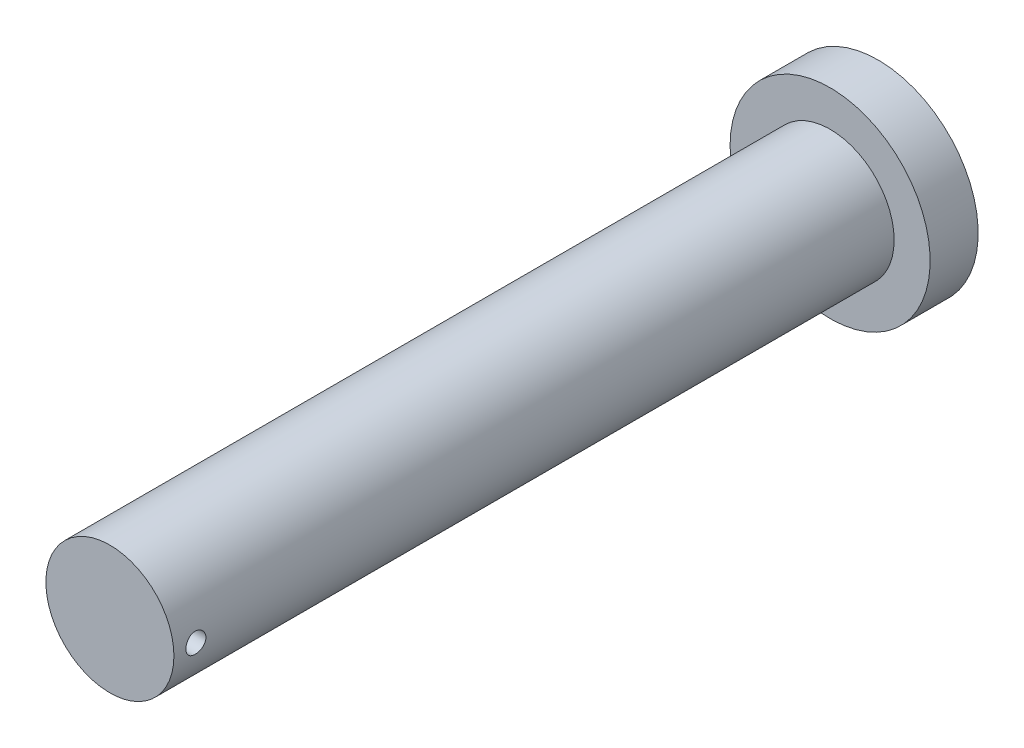
ISO-10303-21;
HEADER;
FILE_DESCRIPTION(('STEP AP214'),'2;1');
FILE_NAME('part.step','',(''),(''),'','','');
FILE_SCHEMA(('AUTOMOTIVE_DESIGN { 1 0 10303 214 1 1 1 1 }'));
ENDSEC;
DATA;
#1=APPLICATION_CONTEXT('core data for automotive mechanical design processes');
#2=APPLICATION_PROTOCOL_DEFINITION('international standard','automotive_design',2000,#1);
#3=PRODUCT_CONTEXT('',#1,'mechanical');
#4=PRODUCT('Part','Part','',(#3));
#5=PRODUCT_RELATED_PRODUCT_CATEGORY('part','',(#4));
#6=PRODUCT_DEFINITION_FORMATION('','',#4);
#7=PRODUCT_DEFINITION_CONTEXT('part definition',#1,'design');
#8=PRODUCT_DEFINITION('design','',#6,#7);
#9=PRODUCT_DEFINITION_SHAPE('','',#8);
#10=(LENGTH_UNIT() NAMED_UNIT(*) SI_UNIT(.MILLI.,.METRE.));
#11=(NAMED_UNIT(*) PLANE_ANGLE_UNIT() SI_UNIT($,.RADIAN.));
#12=(NAMED_UNIT(*) SI_UNIT($,.STERADIAN.) SOLID_ANGLE_UNIT());
#13=UNCERTAINTY_MEASURE_WITH_UNIT(LENGTH_MEASURE(1.E-05),#10,'distance_accuracy_value','');
#14=(GEOMETRIC_REPRESENTATION_CONTEXT(3) GLOBAL_UNCERTAINTY_ASSIGNED_CONTEXT((#13)) GLOBAL_UNIT_ASSIGNED_CONTEXT((#10,
#11,#12)) REPRESENTATION_CONTEXT('',''));
#15=CARTESIAN_POINT('',(0.,0.,0.));
#16=DIRECTION('',(0.,0.,1.));
#17=DIRECTION('',(1.,0.,0.));
#18=AXIS2_PLACEMENT_3D('',#15,#16,#17);
#19=CARTESIAN_POINT('',(0.,0.,180.));
#20=DIRECTION('',(0.,0.,-1.));
#21=DIRECTION('',(-1.,0.,0.));
#22=AXIS2_PLACEMENT_3D('',#19,#20,#21);
#23=CYLINDRICAL_SURFACE('',#22,16.);
#24=CARTESIAN_POINT('',(-16.,0.,177.));
#25=CARTESIAN_POINT('',(-15.9999977019448,-0.139515097271031,176.999994301728));
#26=CARTESIAN_POINT('',(-15.9981561248574,-0.279109404865701,176.988281886226));
#27=CARTESIAN_POINT('',(-15.9909869809759,-0.5543913149781,176.941756308723));
#28=CARTESIAN_POINT('',(-15.9856560884472,-0.690075061323317,176.906921107496));
#29=CARTESIAN_POINT('',(-15.9721069716578,-0.953512538047404,176.815220337193));
#30=CARTESIAN_POINT('',(-15.9638909956317,-1.0812723522899,176.758371918638));
#31=CARTESIAN_POINT('',(-15.9454779403815,-1.3254212510446,176.624301454858));
#32=CARTESIAN_POINT('',(-15.9352811186255,-1.44181181036831,176.547082056964));
#33=CARTESIAN_POINT('',(-15.9139426841436,-1.66091991165161,176.373766951646));
#34=CARTESIAN_POINT('',(-15.9027945139234,-1.76352747914263,176.27753300511));
#35=CARTESIAN_POINT('',(-15.8808607613029,-1.95120768822822,176.069218051731));
#36=CARTESIAN_POINT('',(-15.8700752005075,-2.03627928654191,175.9571361027));
#37=CARTESIAN_POINT('',(-15.8500242812745,-2.18690544328884,175.719561728656));
#38=CARTESIAN_POINT('',(-15.840767397861,-2.25235273557992,175.594000517638));
#39=CARTESIAN_POINT('',(-15.8249120174236,-2.36118681597065,175.333498589142));
#40=CARTESIAN_POINT('',(-15.8183133630222,-2.40457491010064,175.198558427489));
#41=CARTESIAN_POINT('',(-15.8085863451104,-2.46771559322167,174.924289098856));
#42=CARTESIAN_POINT('',(-15.8054302653236,-2.48765705487495,174.785004414181));
#43=CARTESIAN_POINT('',(-15.8028617107177,-2.50392369757621,174.505032811107));
#44=CARTESIAN_POINT('',(-15.8034490028802,-2.50025034860465,174.364345980534));
#45=CARTESIAN_POINT('',(-15.8082755045521,-2.4695458080889,174.086902968147));
#46=CARTESIAN_POINT('',(-15.8124817218495,-2.44272562959693,173.950122776647));
#47=CARTESIAN_POINT('',(-15.8240205634547,-2.36681937833751,173.683027993641));
#48=CARTESIAN_POINT('',(-15.8313532830641,-2.31773262684131,173.552713599359));
#49=CARTESIAN_POINT('',(-15.8483550685462,-2.19846916949384,173.301611287323));
#50=CARTESIAN_POINT('',(-15.8580339308724,-2.12820372315549,173.180866208227));
#51=CARTESIAN_POINT('',(-15.878630461501,-1.96864058146638,172.952800464314));
#52=CARTESIAN_POINT('',(-15.8895482178821,-1.87934153253017,172.845480755113));
#53=CARTESIAN_POINT('',(-15.911537862489,-1.68309088822334,172.646089753367));
#54=CARTESIAN_POINT('',(-15.9226101363559,-1.5759580056054,172.554196841731));
#55=CARTESIAN_POINT('',(-15.9435512534783,-1.34769694737936,172.38966685436));
#56=CARTESIAN_POINT('',(-15.9534200906202,-1.22656870068131,172.317029876443));
#57=CARTESIAN_POINT('',(-15.9708539902704,-0.973595927056479,172.193061926578));
#58=CARTESIAN_POINT('',(-15.9784174854193,-0.841744186240451,172.141745441467));
#59=CARTESIAN_POINT('',(-15.9903756000068,-0.571149534696758,172.062034032553));
#60=CARTESIAN_POINT('',(-15.9947704520898,-0.432407130687203,172.033637425934));
#61=CARTESIAN_POINT('',(-15.9998651172728,-0.153508336763742,172.00081072355));
#62=CARTESIAN_POINT('',(-16.0006027179286,-0.0133814615087077,171.996135521024));
#63=CARTESIAN_POINT('',(-15.9984028649127,0.265654546411639,172.010232705336));
#64=CARTESIAN_POINT('',(-15.9954655349964,0.404563719925156,172.029004302589));
#65=CARTESIAN_POINT('',(-15.9862692369322,0.676473446265708,172.08925838768));
#66=CARTESIAN_POINT('',(-15.9800278421539,0.809501262056046,172.130620758268));
#67=CARTESIAN_POINT('',(-15.9649207568356,1.06673406785663,172.234755094399));
#68=CARTESIAN_POINT('',(-15.9560549341007,1.19093861303941,172.297528138443));
#69=CARTESIAN_POINT('',(-15.9365897274094,1.42807220225041,172.443271991127));
#70=CARTESIAN_POINT('',(-15.9259772866342,1.54090512378372,172.52639742009));
#71=CARTESIAN_POINT('',(-15.9042388046444,1.75110696507806,172.710272085908));
#72=CARTESIAN_POINT('',(-15.8931127309268,1.84847490447018,172.811022439205));
#73=CARTESIAN_POINT('',(-15.8714802753665,2.02588080776691,173.028381197217));
#74=CARTESIAN_POINT('',(-15.860980411908,2.10575398584127,173.145124847122));
#75=CARTESIAN_POINT('',(-15.8419069280583,2.2447556772664,173.390516073661));
#76=CARTESIAN_POINT('',(-15.83333325222,2.30388478778105,173.519163307489));
#77=CARTESIAN_POINT('',(-15.8191307135236,2.39946771944994,173.784229640714));
#78=CARTESIAN_POINT('',(-15.8134908234896,2.43600654947912,173.920617468766));
#79=CARTESIAN_POINT('',(-15.8057657028079,2.48564122040535,174.197689143664));
#80=CARTESIAN_POINT('',(-15.8036802038444,2.49873883084997,174.338372665419));
#81=CARTESIAN_POINT('',(-15.8033105804488,2.50107452690756,174.618398715907));
#82=CARTESIAN_POINT('',(-15.804985160429,2.49057180548425,174.757739096933));
#83=CARTESIAN_POINT('',(-15.8118569894183,2.446562232559,175.032645297144));
#84=CARTESIAN_POINT('',(-15.8170542307995,2.4130554308696,175.168211124502));
#85=CARTESIAN_POINT('',(-15.8303708885491,2.32408329891851,175.43163782664));
#86=CARTESIAN_POINT('',(-15.8384876895341,2.26863761738581,175.559505478258));
#87=CARTESIAN_POINT('',(-15.856731840474,2.13738768546417,175.804165613676));
#88=CARTESIAN_POINT('',(-15.8668592701083,2.06158262820885,175.920957658288));
#89=CARTESIAN_POINT('',(-15.8881156809226,1.89083008139078,176.141465544127));
#90=CARTESIAN_POINT('',(-15.8992540116029,1.79569107094768,176.245032196614));
#91=CARTESIAN_POINT('',(-15.9212004364073,1.58937594638204,176.434821236387));
#92=CARTESIAN_POINT('',(-15.9320084534012,1.47819612078432,176.521039598592));
#93=CARTESIAN_POINT('',(-15.952151024567,1.2421668588434,176.674151223032));
#94=CARTESIAN_POINT('',(-15.9614763443027,1.11723937214236,176.74092537276));
#95=CARTESIAN_POINT('',(-15.9775125983888,0.85785188235777,176.852440996193));
#96=CARTESIAN_POINT('',(-15.9842262014212,0.723401776581757,176.897204972558));
#97=CARTESIAN_POINT('',(-15.9927744586488,0.490314239911593,176.953433021091));
#98=CARTESIAN_POINT('',(-15.9954699162612,0.393105575651622,176.970868490629));
#99=CARTESIAN_POINT('',(-15.9990834869762,0.197277797850579,176.994153913379));
#100=CARTESIAN_POINT('',(-16.0000016250796,0.0986587041691173,177.000004029557));
#101=CARTESIAN_POINT('',(-16.,0.,177.));
#102=B_SPLINE_CURVE_WITH_KNOTS('',3,(#24,#25,#26,#27,#28,#29,#30,#31,#32,#33,#34,#35,#36,#37,
#38,#39,#40,#41,#42,#43,#44,#45,#46,#47,#48,#49,#50,#51,#52,#53,#54,#55,#56,#57,#58,#59,#60,#61,
#62,#63,#64,#65,#66,#67,#68,#69,#70,#71,#72,#73,#74,#75,#76,#77,#78,#79,#80,#81,#82,#83,#84,#85,
#86,#87,#88,#89,#90,#91,#92,#93,#94,#95,#96,#97,#98,#99,#100,#101),.UNSPECIFIED.,.T.,.F.,(4,2,2,
2,2,2,2,2,2,2,2,2,2,2,2,2,2,2,2,2,2,2,2,2,2,2,2,2,2,2,2,2,2,2,2,2,2,2,4),(0.,0.418184740477487,
0.836768642528015,1.25502707944103,1.67323118792029,2.09459568152197,2.51598523645421,
2.9396377860576,3.36326525009241,3.78345631134992,4.20362121670544,4.61999576022581,
5.03638299651049,5.45453977402344,5.87272629892064,6.29545732334366,6.71819049513826,
7.14121043754564,7.56419931829864,7.98280854005912,8.40140366528355,8.81779444756566,
9.23420620742028,9.6538854146967,10.0735912160141,10.4970948024959,10.9205861964898,
11.3424741039513,11.7643301622929,12.1815758159869,12.5988205661889,13.0156924696662,
13.4325808967134,13.8538201231554,14.275156971423,14.6990230419984,15.1224548565628,
15.4181801635154,15.7139013105871),.UNSPECIFIED.);
#103=CARTESIAN_POINT('',(-16.,0.,177.));
#104=VERTEX_POINT('',#103);
#105=EDGE_CURVE('E41',#104,#104,#102,.T.);
#106=ORIENTED_EDGE('',*,*,#105,.T.);
#107=EDGE_LOOP('',(#106));
#108=FACE_BOUND('',#107,.T.);
#109=CARTESIAN_POINT('',(16.,0.,172.));
#110=CARTESIAN_POINT('',(15.9999977019449,-0.139515097271031,172.000005698272));
#111=CARTESIAN_POINT('',(15.9981561248574,-0.279109404865701,172.011718113774));
#112=CARTESIAN_POINT('',(15.9909869809759,-0.554391314978099,172.058243691277));
#113=CARTESIAN_POINT('',(15.9856560884472,-0.690075061323316,172.093078892503));
#114=CARTESIAN_POINT('',(15.9721069716578,-0.953512538047403,172.184779662807));
#115=CARTESIAN_POINT('',(15.9638909956317,-1.0812723522899,172.241628081362));
#116=CARTESIAN_POINT('',(15.9454779403815,-1.3254212510446,172.375698545142));
#117=CARTESIAN_POINT('',(15.9352811186255,-1.44181181036831,172.452917943036));
#118=CARTESIAN_POINT('',(15.9139426841436,-1.66091991165161,172.626233048354));
#119=CARTESIAN_POINT('',(15.9027945139234,-1.76352747914263,172.72246699489));
#120=CARTESIAN_POINT('',(15.8808607613029,-1.95120768822822,172.930781948269));
#121=CARTESIAN_POINT('',(15.8700752005075,-2.03627928654191,173.0428638973));
#122=CARTESIAN_POINT('',(15.8500242812745,-2.18690544328884,173.280438271344));
#123=CARTESIAN_POINT('',(15.840767397861,-2.25235273557992,173.405999482362));
#124=CARTESIAN_POINT('',(15.8249120174236,-2.36118681597065,173.666501410858));
#125=CARTESIAN_POINT('',(15.8183133630222,-2.40457491010064,173.801441572511));
#126=CARTESIAN_POINT('',(15.8085863451104,-2.46771559322167,174.075710901144));
#127=CARTESIAN_POINT('',(15.8054302653236,-2.48765705487495,174.214995585819));
#128=CARTESIAN_POINT('',(15.8028617107177,-2.50392369757621,174.494967188893));
#129=CARTESIAN_POINT('',(15.8034490028802,-2.50025034860465,174.635654019466));
#130=CARTESIAN_POINT('',(15.8082755045521,-2.4695458080889,174.913097031853));
#131=CARTESIAN_POINT('',(15.8124817218495,-2.44272562959693,175.049877223353));
#132=CARTESIAN_POINT('',(15.8240205634547,-2.36681937833752,175.316972006359));
#133=CARTESIAN_POINT('',(15.8313532830641,-2.31773262684132,175.447286400641));
#134=CARTESIAN_POINT('',(15.8483550685462,-2.19846916949384,175.698388712677));
#135=CARTESIAN_POINT('',(15.8580339308724,-2.1282037231555,175.819133791773));
#136=CARTESIAN_POINT('',(15.878630461501,-1.96864058146639,176.047199535685));
#137=CARTESIAN_POINT('',(15.8895482178821,-1.87934153253018,176.154519244887));
#138=CARTESIAN_POINT('',(15.911537862489,-1.68309088822334,176.353910246633));
#139=CARTESIAN_POINT('',(15.9226101363559,-1.5759580056054,176.445803158269));
#140=CARTESIAN_POINT('',(15.9435512534783,-1.34769694737936,176.61033314564));
#141=CARTESIAN_POINT('',(15.9534200906202,-1.22656870068131,176.682970123557));
#142=CARTESIAN_POINT('',(15.9708539902704,-0.973595927056482,176.806938073422));
#143=CARTESIAN_POINT('',(15.9784174854193,-0.841744186240457,176.858254558533));
#144=CARTESIAN_POINT('',(15.9903756000068,-0.571149534696764,176.937965967447));
#145=CARTESIAN_POINT('',(15.9947704520898,-0.432407130687207,176.966362574066));
#146=CARTESIAN_POINT('',(15.9998651172728,-0.153508336763743,176.99918927645));
#147=CARTESIAN_POINT('',(16.0006027179286,-0.0133814615087094,177.003864478976));
#148=CARTESIAN_POINT('',(15.9984028649127,0.265654546411637,176.989767294664));
#149=CARTESIAN_POINT('',(15.9954655349964,0.404563719925154,176.970995697411));
#150=CARTESIAN_POINT('',(15.9862692369322,0.676473446265707,176.91074161232));
#151=CARTESIAN_POINT('',(15.9800278421539,0.809501262056046,176.869379241732));
#152=CARTESIAN_POINT('',(15.9649207568356,1.06673406785663,176.765244905601));
#153=CARTESIAN_POINT('',(15.9560549341007,1.19093861303941,176.702471861557));
#154=CARTESIAN_POINT('',(15.9365897274094,1.4280722022504,176.556728008873));
#155=CARTESIAN_POINT('',(15.9259772866342,1.54090512378371,176.47360257991));
#156=CARTESIAN_POINT('',(15.9042388046444,1.75110696507805,176.289727914092));
#157=CARTESIAN_POINT('',(15.8931127309268,1.84847490447017,176.188977560795));
#158=CARTESIAN_POINT('',(15.8714802753665,2.0258808077669,175.971618802783));
#159=CARTESIAN_POINT('',(15.860980411908,2.10575398584125,175.854875152878));
#160=CARTESIAN_POINT('',(15.8419069280583,2.24475567726639,175.609483926339));
#161=CARTESIAN_POINT('',(15.83333325222,2.30388478778104,175.480836692511));
#162=CARTESIAN_POINT('',(15.8191307135236,2.39946771944994,175.215770359286));
#163=CARTESIAN_POINT('',(15.8134908234896,2.43600654947912,175.079382531234));
#164=CARTESIAN_POINT('',(15.8057657028079,2.48564122040535,174.802310856336));
#165=CARTESIAN_POINT('',(15.8036802038444,2.49873883084997,174.661627334581));
#166=CARTESIAN_POINT('',(15.8033105804488,2.50107452690756,174.381601284093));
#167=CARTESIAN_POINT('',(15.804985160429,2.49057180548425,174.242260903066));
#168=CARTESIAN_POINT('',(15.8118569894183,2.446562232559,173.967354702856));
#169=CARTESIAN_POINT('',(15.8170542307995,2.41305543086961,173.831788875498));
#170=CARTESIAN_POINT('',(15.8303708885491,2.32408329891851,173.56836217336));
#171=CARTESIAN_POINT('',(15.8384876895341,2.26863761738581,173.440494521742));
#172=CARTESIAN_POINT('',(15.856731840474,2.13738768546418,173.195834386324));
#173=CARTESIAN_POINT('',(15.8668592701083,2.06158262820885,173.079042341712));
#174=CARTESIAN_POINT('',(15.8881156809226,1.89083008139079,172.858534455873));
#175=CARTESIAN_POINT('',(15.8992540116029,1.79569107094768,172.754967803386));
#176=CARTESIAN_POINT('',(15.9212004364073,1.58937594638204,172.565178763613));
#177=CARTESIAN_POINT('',(15.9320084534012,1.47819612078432,172.478960401408));
#178=CARTESIAN_POINT('',(15.952151024567,1.2421668588434,172.325848776968));
#179=CARTESIAN_POINT('',(15.9614763443027,1.11723937214236,172.25907462724));
#180=CARTESIAN_POINT('',(15.9775125983888,0.857851882357769,172.147559003807));
#181=CARTESIAN_POINT('',(15.9842262014212,0.723401776581757,172.102795027442));
#182=CARTESIAN_POINT('',(15.9927744586488,0.490314239911594,172.046566978909));
#183=CARTESIAN_POINT('',(15.9954699162612,0.393105575651623,172.029131509371));
#184=CARTESIAN_POINT('',(15.9990834869762,0.197277797850579,172.005846086621));
#185=CARTESIAN_POINT('',(16.0000016250797,0.0986587041691174,171.999995970443));
#186=CARTESIAN_POINT('',(16.,0.,172.));
#187=B_SPLINE_CURVE_WITH_KNOTS('',3,(#109,#110,#111,#112,#113,#114,#115,#116,#117,#118,#119,
#120,#121,#122,#123,#124,#125,#126,#127,#128,#129,#130,#131,#132,#133,#134,#135,#136,#137,#138,
#139,#140,#141,#142,#143,#144,#145,#146,#147,#148,#149,#150,#151,#152,#153,#154,#155,#156,#157,
#158,#159,#160,#161,#162,#163,#164,#165,#166,#167,#168,#169,#170,#171,#172,#173,#174,#175,#176,
#177,#178,#179,#180,#181,#182,#183,#184,#185,#186),.UNSPECIFIED.,.T.,.F.,(4,2,2,2,2,2,2,2,2,2,2,
2,2,2,2,2,2,2,2,2,2,2,2,2,2,2,2,2,2,2,2,2,2,2,2,2,2,2,4),(0.,0.418184740477487,
0.836768642528015,1.25502707944103,1.67323118792029,2.09459568152197,2.51598523645421,
2.9396377860576,3.36326525009241,3.78345631134992,4.20362121670544,4.61999576022578,
5.03638299651049,5.45453977402341,5.87272629892064,6.29545732334366,6.71819049513826,
7.14121043754563,7.56419931829864,7.98280854005912,8.40140366528355,8.81779444756566,
9.23420620742028,9.65388541469668,10.0735912160141,10.4970948024958,10.9205861964898,
11.3424741039513,11.7643301622929,12.1815758159869,12.5988205661889,13.0156924696661,
13.4325808967134,13.8538201231554,14.275156971423,14.6990230419984,15.1224548565628,
15.4181801635154,15.7139013105871),.UNSPECIFIED.);
#188=CARTESIAN_POINT('',(16.,0.,172.));
#189=VERTEX_POINT('',#188);
#190=EDGE_CURVE('E56',#189,#189,#187,.T.);
#191=ORIENTED_EDGE('',*,*,#190,.T.);
#192=EDGE_LOOP('',(#191));
#193=FACE_BOUND('',#192,.T.);
#194=CARTESIAN_POINT('',(0.,0.,180.));
#195=DIRECTION('',(0.,0.,1.));
#196=DIRECTION('',(1.,0.,0.));
#197=AXIS2_PLACEMENT_3D('',#194,#195,#196);
#198=CIRCLE('',#197,16.);
#199=CARTESIAN_POINT('',(16.,0.,180.));
#200=VERTEX_POINT('',#199);
#201=EDGE_CURVE('E10',#200,#200,#198,.T.);
#202=ORIENTED_EDGE('',*,*,#201,.F.);
#203=EDGE_LOOP('',(#202));
#204=FACE_BOUND('',#203,.T.);
#205=CARTESIAN_POINT('',(0.,0.,0.));
#206=DIRECTION('',(0.,0.,1.));
#207=DIRECTION('',(1.,0.,0.));
#208=AXIS2_PLACEMENT_3D('',#205,#206,#207);
#209=CIRCLE('',#208,16.);
#210=CARTESIAN_POINT('',(16.,0.,0.));
#211=VERTEX_POINT('',#210);
#212=EDGE_CURVE('E47',#211,#211,#209,.T.);
#213=ORIENTED_EDGE('',*,*,#212,.T.);
#214=EDGE_LOOP('',(#213));
#215=FACE_BOUND('',#214,.T.);
#216=ADVANCED_FACE('F40',(#108,#193,#204,#215),#23,.T.);
#217=CARTESIAN_POINT('',(0.,0.,180.));
#218=DIRECTION('',(0.,0.,1.));
#219=DIRECTION('',(1.,0.,0.));
#220=AXIS2_PLACEMENT_3D('',#217,#218,#219);
#221=PLANE('',#220);
#222=ORIENTED_EDGE('',*,*,#201,.T.);
#223=EDGE_LOOP('',(#222));
#224=FACE_BOUND('',#223,.T.);
#225=ADVANCED_FACE('F79',(#224),#221,.T.);
#226=CARTESIAN_POINT('',(0.,0.,-12.));
#227=DIRECTION('',(0.,0.,1.));
#228=DIRECTION('',(1.,0.,0.));
#229=AXIS2_PLACEMENT_3D('',#226,#227,#228);
#230=CYLINDRICAL_SURFACE('',#229,25.);
#231=CARTESIAN_POINT('',(0.,0.,-12.));
#232=DIRECTION('',(0.,0.,-1.));
#233=DIRECTION('',(-1.,0.,0.));
#234=AXIS2_PLACEMENT_3D('',#231,#232,#233);
#235=CIRCLE('',#234,25.);
#236=CARTESIAN_POINT('',(-25.,0.,-12.));
#237=VERTEX_POINT('',#236);
#238=EDGE_CURVE('E53',#237,#237,#235,.T.);
#239=ORIENTED_EDGE('',*,*,#238,.F.);
#240=EDGE_LOOP('',(#239));
#241=FACE_BOUND('',#240,.T.);
#242=CARTESIAN_POINT('',(0.,0.,0.));
#243=DIRECTION('',(0.,0.,-1.));
#244=DIRECTION('',(-1.,0.,0.));
#245=AXIS2_PLACEMENT_3D('',#242,#243,#244);
#246=CIRCLE('',#245,25.);
#247=CARTESIAN_POINT('',(-25.,0.,0.));
#248=VERTEX_POINT('',#247);
#249=EDGE_CURVE('E60',#248,#248,#246,.T.);
#250=ORIENTED_EDGE('',*,*,#249,.T.);
#251=EDGE_LOOP('',(#250));
#252=FACE_BOUND('',#251,.T.);
#253=ADVANCED_FACE('F74',(#241,#252),#230,.T.);
#254=CARTESIAN_POINT('',(0.,0.,-12.));
#255=DIRECTION('',(0.,0.,-1.));
#256=DIRECTION('',(-1.,0.,0.));
#257=AXIS2_PLACEMENT_3D('',#254,#255,#256);
#258=PLANE('',#257);
#259=ORIENTED_EDGE('',*,*,#238,.T.);
#260=EDGE_LOOP('',(#259));
#261=FACE_BOUND('',#260,.T.);
#262=ADVANCED_FACE('F68',(#261),#258,.T.);
#263=CARTESIAN_POINT('',(0.,0.,0.));
#264=DIRECTION('',(0.,0.,-1.));
#265=DIRECTION('',(-1.,0.,0.));
#266=AXIS2_PLACEMENT_3D('',#263,#264,#265);
#267=PLANE('',#266);
#268=ORIENTED_EDGE('',*,*,#212,.F.);
#269=EDGE_LOOP('',(#268));
#270=FACE_BOUND('',#269,.T.);
#271=ORIENTED_EDGE('',*,*,#249,.F.);
#272=EDGE_LOOP('',(#271));
#273=FACE_BOUND('',#272,.T.);
#274=ADVANCED_FACE('F70',(#270,#273),#267,.F.);
#275=CARTESIAN_POINT('',(-75.,0.,174.5));
#276=DIRECTION('',(1.,0.,0.));
#277=DIRECTION('',(0.,0.,-1.));
#278=AXIS2_PLACEMENT_3D('',#275,#276,#277);
#279=CYLINDRICAL_SURFACE('',#278,2.5);
#280=ORIENTED_EDGE('',*,*,#190,.F.);
#281=EDGE_LOOP('',(#280));
#282=FACE_BOUND('',#281,.T.);
#283=ORIENTED_EDGE('',*,*,#105,.F.);
#284=EDGE_LOOP('',(#283));
#285=FACE_BOUND('',#284,.T.);
#286=ADVANCED_FACE('F63',(#282,#285),#279,.F.);
#287=CLOSED_SHELL('',(#216,#225,#253,#262,#274,#286));
#288=MANIFOLD_SOLID_BREP('B2',#287);
#289=ADVANCED_BREP_SHAPE_REPRESENTATION('',(#18,#288),#14);
#290=SHAPE_DEFINITION_REPRESENTATION(#9,#289);
ENDSEC;
END-ISO-10303-21;
